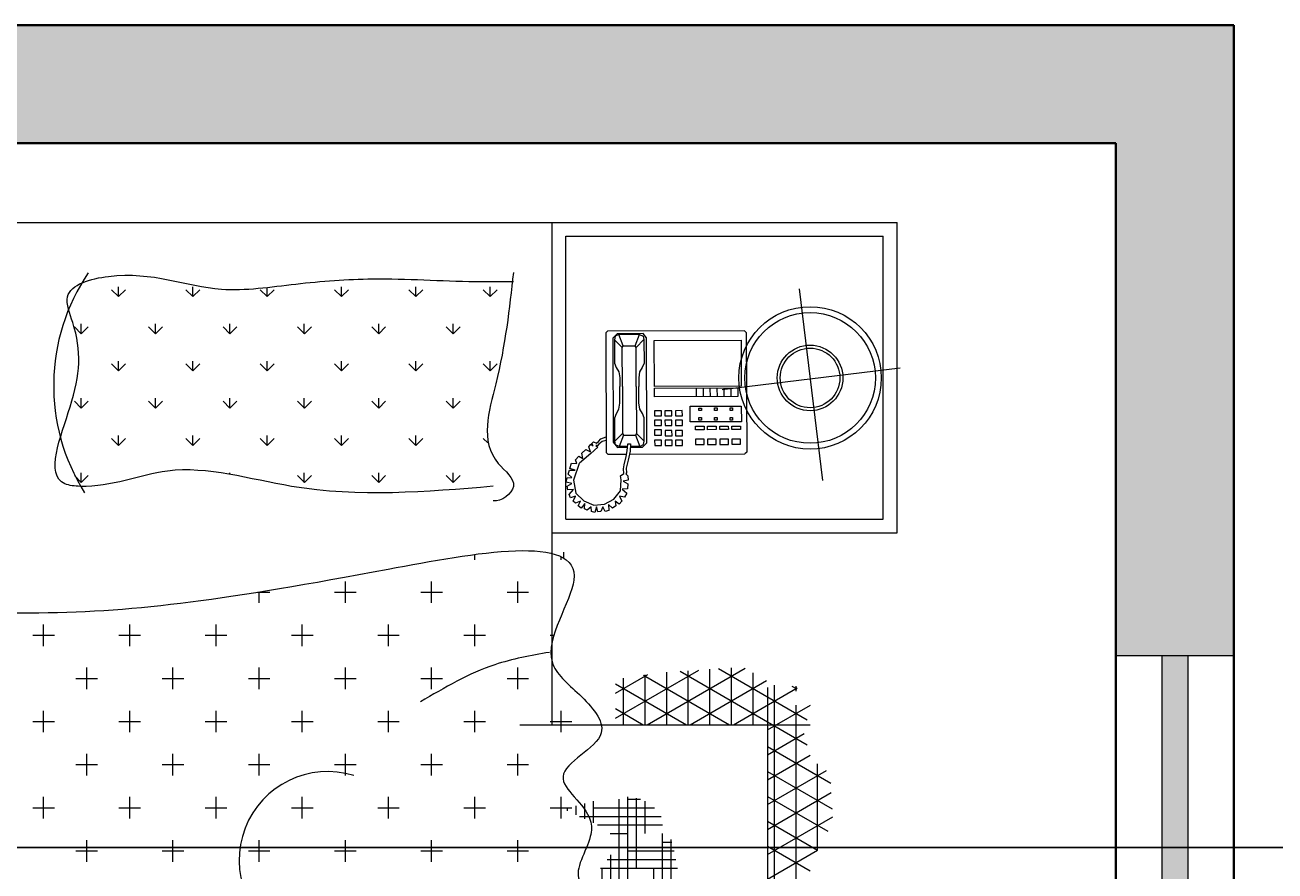
# Model space of a CAD drawing. Units: inches. Extents: x 2330 to 3943, y 1763 to 3461.
# Tile 37 of 40: x 3364 to 3459, y 3098 to 3163. Entities that reach past the tile are written whole.
import ezdxf

# ---------------------------------------------------------------- set-up
doc = ezdxf.new("R2010")
doc.units = ezdxf.units.IN
for name, color, linetype, lineweight in [('A-ANNO-DIMS', 2, 'Continuous', 18), ('A-FURN', 8, 'Continuous', 13), ('A-GLAZ', 4, 'Continuous', 18), ('A-WALL', 7, 'Continuous', 40), ('A-WALL-PATT', 252, 'Continuous', 13)]:
    doc.layers.add(name, color=color, linetype=linetype, lineweight=lineweight)
doc.styles.get("Standard").update_dxf_attribs({"font": 'arial.ttf'})
doc.dimstyles.get("Standard").update_dxf_attribs({"dimtxt": 0.18, "dimasz": 0.18, "dimexe": 0.18, "dimexo": 0.0625, "dimgap": 0.09, "dimtad": 0, "dimtih": 1, "dimtoh": 1, "dimdec": 4, "dimzin": 0, "dimdsep": 46, "dimtxsty": 'Standard', "dimcen": 0.09, "dimadec": 0, "dimazin": 0, "dimtfac": 1, "dimtdec": 4, "dimtofl": 0, "dimtmove": 0, "dimatfit": 3, "dimfxl": 1, "dimtolj": 1, "dimtzin": 0, "dimarcsym": 0})

# ---------------------------------------------------------------- blocks, each defined once
blk = doc.blocks.new('A$C200C7901')
for p, q in [((0.5, 2.3334), (2, 2.3334)), ((2, 2.3334), (2.5, 2.3334)), ((2, 1.6055), (2, 2.3334)), ((2.5, 1.8834), (2.5, 2.3334)), ((1.3176, 2.1721), (1.3075, 2.1822)), ((1.3176, 2.1721), (1.3075, 2.1822)), ((2, 1.8834), (2.5, 1.8834)), ((2.0129, 1.8445), (2.0129, 1.849)), ((2.0129, 1.8445), (2.0129, 1.849)), ((2.0171, 1.8467), (2.0171, 1.8556)), ((2.0171, 1.8467), (2.0171, 1.8556)), ((1.9972, 1.7352), (2.0027, 1.7352)), ((1.9972, 1.7352), (2.0027, 1.7352)), ((2, 1.6963), (2, 1.7248)), ((2, 1.6963), (2, 1.7248)), ((2.3121, 1.6596), (2.3121, 0.0201)), ((1.9533, 1.6055), (2.3741, 1.6055)), ((1.9533, 1.6055), (2.3741, 1.6055))]:
    blk.add_line(p, q)
at = {"linetype": 'ByBlock'}
for p, q in [((2.02, 2.3134), (2.48, 2.3134)), ((2.02, 1.9034), (2.02, 2.3134)), ((2.48, 1.9034), (2.48, 2.3134)), ((1.3714, 2.2259), (1.3613, 2.236)), ((1.3714, 2.2259), (1.3613, 2.236)), ((1.3714, 2.2259), (1.3714, 2.2402)), ((1.3714, 2.2259), (1.3714, 2.2402)), ((1.3714, 2.2259), (1.3815, 2.236)), ((1.3714, 2.2259), (1.3815, 2.236)), ((1.4792, 2.2259), (1.4691, 2.236)), ((1.4792, 2.2259), (1.4691, 2.236)), ((1.4792, 2.2259), (1.4792, 2.2402)), ((1.4792, 2.2259), (1.4792, 2.2402)), ((1.4792, 2.2259), (1.4893, 2.236)), ((1.4792, 2.2259), (1.4893, 2.236)), ((1.587, 2.2259), (1.5769, 2.236)), ((1.587, 2.2259), (1.5769, 2.236)), ((1.587, 2.2259), (1.587, 2.2393)), ((1.587, 2.2259), (1.587, 2.2393)), ((1.587, 2.2259), (1.5971, 2.236)), ((1.587, 2.2259), (1.5971, 2.236)), ((1.6947, 2.2259), (1.6846, 2.236)), ((1.6947, 2.2259), (1.6846, 2.236)), ((1.6947, 2.2259), (1.6947, 2.2402)), ((1.6947, 2.2259), (1.6947, 2.2402)), ((1.6947, 2.2259), (1.7048, 2.236)), ((1.6947, 2.2259), (1.7048, 2.236)), ((1.8025, 2.2259), (1.7924, 2.236)), ((1.8025, 2.2259), (1.7924, 2.236)), ((1.8025, 2.2259), (1.8025, 2.2402)), ((1.8025, 2.2259), (1.8025, 2.2402)), ((1.8025, 2.2259), (1.8126, 2.236)), ((1.8025, 2.2259), (1.8126, 2.236)), ((1.9103, 2.2259), (1.9002, 2.236)), ((1.9103, 2.2259), (1.9002, 2.236)), ((1.9103, 2.2259), (1.9103, 2.2402)), ((1.9103, 2.2259), (1.9103, 2.2402)), ((1.9103, 2.2259), (1.9204, 2.236)), ((1.9103, 2.2259), (1.9204, 2.236)), ((2.3581, 2.2373), (2.3919, 1.9595)), ((1.3176, 2.172), (1.3176, 2.1863)), ((1.3176, 2.172), (1.3176, 2.1863)), ((1.3176, 2.1721), (1.3277, 2.1822)), ((1.3176, 2.1721), (1.3277, 2.1822)), ((1.4253, 2.1721), (1.4152, 2.1822)), ((1.4253, 2.1721), (1.4152, 2.1822)), ((1.4253, 2.172), (1.4253, 2.1863)), ((1.4253, 2.172), (1.4253, 2.1863)), ((1.4253, 2.1721), (1.4354, 2.1822)), ((1.4253, 2.1721), (1.4354, 2.1822)), ((1.5331, 2.1721), (1.523, 2.1822)), ((1.5331, 2.1721), (1.523, 2.1822)), ((1.5331, 2.172), (1.5331, 2.1863)), ((1.5331, 2.172), (1.5331, 2.1863)), ((1.5331, 2.1721), (1.5432, 2.1822)), ((1.5331, 2.1721), (1.5432, 2.1822)), ((1.6409, 2.1721), (1.6308, 2.1822)), ((1.6409, 2.1721), (1.6308, 2.1822)), ((1.6408, 2.172), (1.6408, 2.1863)), ((1.6408, 2.172), (1.6408, 2.1863)), ((1.6409, 2.1721), (1.651, 2.1822)), ((1.6409, 2.1721), (1.651, 2.1822)), ((1.7486, 2.1721), (1.7385, 2.1822)), ((1.7486, 2.1721), (1.7385, 2.1822)), ((1.7486, 2.172), (1.7486, 2.1863)), ((1.7486, 2.172), (1.7486, 2.1863)), ((1.7486, 2.1721), (1.7587, 2.1822)), ((1.7486, 2.1721), (1.7587, 2.1822)), ((1.8564, 2.1721), (1.8463, 2.1822)), ((1.8564, 2.1721), (1.8463, 2.1822)), ((1.8564, 2.172), (1.8564, 2.1863)), ((1.8564, 2.172), (1.8564, 2.1863)), ((1.8564, 2.1721), (1.8665, 2.1822)), ((1.8564, 2.1721), (1.8665, 2.1822)), ((2.0802, 2.176), (2.0777, 2.1734)), ((2.2789, 2.1766), (2.0802, 2.176)), ((2.2789, 2.1766), (2.2814, 2.1741)), ((2.0777, 2.1734), (2.0783, 1.9999)), ((2.0941, 2.1722), (2.0878, 2.1659)), ((2.0878, 2.1659), (2.0883, 2.015)), ((2.0915, 2.1685), (2.0903, 2.1634)), ((2.0903, 2.1634), (2.1017, 2.1521)), ((2.0903, 2.1634), (2.0904, 2.1295)), ((2.0966, 2.171), (2.0915, 2.1685)), ((2.1318, 2.1724), (2.0941, 2.1722)), ((2.1267, 2.1711), (2.0966, 2.171)), ((2.1029, 2.1547), (2.0966, 2.171)), ((2.1205, 2.1547), (2.1267, 2.1711)), ((2.1331, 2.1636), (2.1218, 2.1522)), ((2.1267, 2.1711), (2.1318, 2.1686)), ((2.1368, 2.1661), (2.1318, 2.1724)), ((2.1318, 2.1686), (2.1331, 2.1636)), ((2.1331, 2.1636), (2.1332, 2.1296)), ((2.1373, 2.014), (2.1368, 2.1661)), ((2.1481, 2.1624), (2.2739, 2.1628)), ((2.1484, 2.0957), (2.1481, 2.1624)), ((2.2739, 2.1628), (2.2741, 2.0961)), ((2.2814, 2.1741), (2.282, 2.0006)), ((2.1017, 2.1521), (2.1029, 2.1547)), ((2.1019, 2.0956), (2.1017, 2.1521)), ((2.1029, 2.1547), (2.1205, 2.1547)), ((2.1218, 2.1522), (2.1205, 2.1547)), ((2.122, 2.0956), (2.1218, 2.1522)), ((1.3714, 2.1182), (1.3613, 2.1283)), ((1.3714, 2.1182), (1.3613, 2.1283)), ((1.3714, 2.1182), (1.3714, 2.1325)), ((1.3714, 2.1182), (1.3714, 2.1325)), ((1.3714, 2.1182), (1.3815, 2.1283)), ((1.3714, 2.1182), (1.3815, 2.1283)), ((1.4792, 2.1182), (1.4691, 2.1283)), ((1.4792, 2.1182), (1.4691, 2.1283)), ((1.4792, 2.1182), (1.4792, 2.1325)), ((1.4792, 2.1182), (1.4792, 2.1325)), ((1.4792, 2.1182), (1.4893, 2.1283)), ((1.4792, 2.1182), (1.4893, 2.1283)), ((1.587, 2.1182), (1.5769, 2.1283)), ((1.587, 2.1182), (1.5769, 2.1283)), ((1.587, 2.1182), (1.587, 2.1325)), ((1.587, 2.1182), (1.587, 2.1325)), ((1.587, 2.1182), (1.5971, 2.1283)), ((1.587, 2.1182), (1.5971, 2.1283)), ((1.6947, 2.1182), (1.6846, 2.1283)), ((1.6947, 2.1182), (1.6846, 2.1283)), ((1.6947, 2.1182), (1.6947, 2.1325)), ((1.6947, 2.1182), (1.6947, 2.1325)), ((1.6947, 2.1182), (1.7048, 2.1283)), ((1.6947, 2.1182), (1.7048, 2.1283)), ((1.8025, 2.1182), (1.7924, 2.1283)), ((1.8025, 2.1182), (1.7924, 2.1283)), ((1.8025, 2.1182), (1.8025, 2.1325)), ((1.8025, 2.1182), (1.8025, 2.1325)), ((1.8025, 2.1182), (1.8126, 2.1283)), ((1.8025, 2.1182), (1.8126, 2.1283)), ((1.9103, 2.1182), (1.9002, 2.1283)), ((1.9103, 2.1182), (1.9002, 2.1283)), ((1.9103, 2.1182), (1.9103, 2.1325)), ((1.9103, 2.1182), (1.9103, 2.1325)), ((1.9103, 2.1182), (1.9204, 2.1283)), ((1.9103, 2.1182), (1.9204, 2.1283)), ((2.0904, 2.1295), (2.093, 2.1232)), ((2.093, 2.1232), (2.0968, 2.1169)), ((2.1307, 2.1233), (2.1269, 2.117)), ((2.1332, 2.1296), (2.1307, 2.1233)), ((2.2464, 2.0911), (2.5044, 2.1228)), ((2.0968, 2.1169), (2.098, 2.1081)), ((2.098, 2.1081), (2.0981, 2.0956)), ((2.1269, 2.117), (2.1257, 2.1082)), ((2.1257, 2.1082), (2.1257, 2.0956)), ((2.0982, 2.0717), (2.0981, 2.0956)), ((2.1019, 2.0956), (2.1021, 2.0277)), ((2.122, 2.0956), (2.1222, 2.0277)), ((2.1258, 2.0718), (2.1257, 2.0956)), ((2.2741, 2.0961), (2.1484, 2.0957)), ((2.1484, 2.0932), (2.2691, 2.0936)), ((2.1484, 2.0806), (2.1484, 2.0932)), ((2.2087, 2.0934), (2.2088, 2.0808)), ((2.2188, 2.0934), (2.2188, 2.0809)), ((2.2288, 2.0935), (2.2289, 2.0809)), ((2.2389, 2.0935), (2.239, 2.0809)), ((2.249, 2.0935), (2.249, 2.081)), ((2.259, 2.0936), (2.2591, 2.081)), ((2.2691, 2.0936), (2.2691, 2.081)), ((1.3176, 2.0643), (1.3075, 2.0744)), ((1.3176, 2.0643), (1.3075, 2.0744)), ((1.3176, 2.0643), (1.3176, 2.0786)), ((1.3176, 2.0643), (1.3176, 2.0786)), ((1.3176, 2.0643), (1.3277, 2.0744)), ((1.3176, 2.0643), (1.3277, 2.0744)), ((1.4253, 2.0643), (1.4152, 2.0744)), ((1.4253, 2.0643), (1.4152, 2.0744)), ((1.4253, 2.0643), (1.4253, 2.0786)), ((1.4253, 2.0643), (1.4253, 2.0786)), ((1.4253, 2.0643), (1.4354, 2.0744)), ((1.4253, 2.0643), (1.4354, 2.0744)), ((1.5331, 2.0643), (1.523, 2.0744)), ((1.5331, 2.0643), (1.523, 2.0744)), ((1.5331, 2.0643), (1.5331, 2.0786)), ((1.5331, 2.0643), (1.5331, 2.0786)), ((1.5331, 2.0643), (1.5432, 2.0744)), ((1.5331, 2.0643), (1.5432, 2.0744)), ((1.6409, 2.0643), (1.6308, 2.0744)), ((1.6409, 2.0643), (1.6308, 2.0744)), ((1.6408, 2.0643), (1.6408, 2.0786)), ((1.6408, 2.0643), (1.6408, 2.0786)), ((1.6409, 2.0643), (1.651, 2.0744)), ((1.6409, 2.0643), (1.651, 2.0744)), ((1.7486, 2.0643), (1.7385, 2.0744)), ((1.7486, 2.0643), (1.7385, 2.0744)), ((1.7486, 2.0643), (1.7486, 2.0786)), ((1.7486, 2.0643), (1.7486, 2.0786)), ((1.7486, 2.0643), (1.7587, 2.0744)), ((1.7486, 2.0643), (1.7587, 2.0744)), ((1.8564, 2.0643), (1.8463, 2.0744)), ((1.8564, 2.0643), (1.8463, 2.0744)), ((1.8564, 2.0643), (1.8564, 2.0786)), ((1.8564, 2.0643), (1.8564, 2.0786)), ((1.8564, 2.0643), (1.8665, 2.0744)), ((1.8564, 2.0643), (1.8665, 2.0744)), ((2.0969, 2.0629), (2.0982, 2.0717)), ((2.1271, 2.063), (2.1258, 2.0718)), ((2.2691, 2.081), (2.1484, 2.0806)), ((2.2, 2.067), (2.2742, 2.0672)), ((2.2001, 2.0443), (2.2, 2.067)), ((2.2742, 2.0672), (2.2743, 2.0446)), ((2.0907, 2.0503), (2.0932, 2.0566)), ((2.0908, 2.0163), (2.0907, 2.0503)), ((2.0932, 2.0566), (2.0969, 2.0629)), ((2.1309, 2.0567), (2.1271, 2.063)), ((2.1334, 2.0504), (2.1309, 2.0567)), ((2.1336, 2.0165), (2.1334, 2.0504)), ((2.1586, 2.0606), (2.1485, 2.0605)), ((2.1485, 2.0605), (2.1485, 2.053)), ((2.1485, 2.053), (2.1586, 2.053)), ((2.1586, 2.053), (2.1586, 2.0606)), ((2.1636, 2.0606), (2.1636, 2.053)), ((2.1736, 2.0606), (2.1636, 2.0606)), ((2.1636, 2.053), (2.1737, 2.0531)), ((2.1737, 2.0531), (2.1736, 2.0606)), ((2.1887, 2.0607), (2.1787, 2.0606)), ((2.1787, 2.0606), (2.1787, 2.0531)), ((2.1787, 2.0531), (2.1888, 2.0531)), ((2.1888, 2.0531), (2.1887, 2.0607)), ((2.2126, 2.0645), (2.2164, 2.0645)), ((2.2126, 2.0607), (2.2126, 2.0645)), ((2.2164, 2.0607), (2.2126, 2.0607)), ((2.2126, 2.0507), (2.2164, 2.0507)), ((2.2127, 2.0469), (2.2126, 2.0507)), ((2.2164, 2.0645), (2.2164, 2.0607)), ((2.2164, 2.0507), (2.2164, 2.0469)), ((2.2352, 2.0646), (2.239, 2.0646)), ((2.2352, 2.0608), (2.2352, 2.0646)), ((2.239, 2.0608), (2.2352, 2.0608)), ((2.2353, 2.0508), (2.2391, 2.0508)), ((2.2353, 2.047), (2.2353, 2.0508)), ((2.239, 2.0646), (2.239, 2.0608)), ((2.2391, 2.0508), (2.2391, 2.047)), ((2.2579, 2.0609), (2.2579, 2.0647)), ((2.2579, 2.0647), (2.2616, 2.0647)), ((2.2616, 2.0609), (2.2579, 2.0609)), ((2.2579, 2.0508), (2.2617, 2.0508)), ((2.2579, 2.0471), (2.2579, 2.0508)), ((2.2616, 2.0647), (2.2616, 2.0609)), ((2.2617, 2.0508), (2.2617, 2.0471)), ((2.1485, 2.0467), (2.1486, 2.0391)), ((2.1586, 2.0467), (2.1485, 2.0467)), ((2.1486, 2.0391), (2.1586, 2.0392)), ((2.1586, 2.0329), (2.1486, 2.0329)), ((2.1486, 2.0329), (2.1486, 2.0253)), ((2.1586, 2.0392), (2.1586, 2.0467)), ((2.1587, 2.0253), (2.1586, 2.0329)), ((2.1737, 2.0468), (2.1636, 2.0467)), ((2.1636, 2.0467), (2.1637, 2.0392)), ((2.1637, 2.0392), (2.1737, 2.0392)), ((2.1637, 2.0317), (2.1637, 2.0241)), ((2.1737, 2.0317), (2.1637, 2.0317)), ((2.1737, 2.0392), (2.1737, 2.0468)), ((2.1738, 2.0241), (2.1737, 2.0317)), ((2.1787, 2.0468), (2.1787, 2.0392)), ((2.1888, 2.0468), (2.1787, 2.0468)), ((2.1787, 2.0392), (2.1888, 2.0393)), ((2.1788, 2.0317), (2.1788, 2.0242)), ((2.1888, 2.0317), (2.1788, 2.0317)), ((2.1888, 2.0393), (2.1888, 2.0468)), ((2.1889, 2.0242), (2.1888, 2.0317)), ((2.2743, 2.0446), (2.2001, 2.0443)), ((2.2077, 2.0331), (2.2077, 2.0381)), ((2.2077, 2.0381), (2.2202, 2.0381)), ((2.2203, 2.0331), (2.2077, 2.0331)), ((2.2164, 2.0469), (2.2127, 2.0469)), ((2.2202, 2.0381), (2.2203, 2.0331)), ((2.2253, 2.0381), (2.2378, 2.0382)), ((2.2253, 2.0331), (2.2253, 2.0381)), ((2.2379, 2.0332), (2.2253, 2.0331)), ((2.2391, 2.047), (2.2353, 2.047)), ((2.2378, 2.0382), (2.2379, 2.0332)), ((2.2429, 2.0332), (2.2429, 2.0382)), ((2.2429, 2.0382), (2.2554, 2.0382)), ((2.2555, 2.0332), (2.2429, 2.0332)), ((2.2554, 2.0382), (2.2555, 2.0332)), ((2.2617, 2.0471), (2.2579, 2.0471)), ((2.2605, 2.0332), (2.2605, 2.0383)), ((2.2605, 2.0383), (2.273, 2.0383)), ((2.2731, 2.0333), (2.2605, 2.0332)), ((2.273, 2.0383), (2.2731, 2.0333)), ((1.3714, 2.0104), (1.3613, 2.0205)), ((1.3714, 2.0104), (1.3613, 2.0205)), ((1.3714, 2.0104), (1.3714, 2.0247)), ((1.3714, 2.0104), (1.3714, 2.0247)), ((1.3714, 2.0104), (1.3815, 2.0205)), ((1.3714, 2.0104), (1.3815, 2.0205)), ((1.4792, 2.0104), (1.4691, 2.0205)), ((1.4792, 2.0104), (1.4691, 2.0205)), ((1.4792, 2.0104), (1.4792, 2.0247)), ((1.4792, 2.0104), (1.4792, 2.0247)), ((1.4792, 2.0104), (1.4893, 2.0205)), ((1.4792, 2.0104), (1.4893, 2.0205)), ((1.587, 2.0104), (1.5769, 2.0205)), ((1.587, 2.0104), (1.5769, 2.0205)), ((1.587, 2.0104), (1.587, 2.0247)), ((1.587, 2.0104), (1.587, 2.0247)), ((1.587, 2.0104), (1.5971, 2.0205)), ((1.587, 2.0104), (1.5971, 2.0205)), ((1.6947, 2.0104), (1.6846, 2.0205)), ((1.6947, 2.0104), (1.6846, 2.0205)), ((1.6947, 2.0104), (1.6947, 2.0247)), ((1.6947, 2.0104), (1.6947, 2.0247)), ((1.6947, 2.0104), (1.7048, 2.0205)), ((1.6947, 2.0104), (1.7048, 2.0205)), ((1.8025, 2.0104), (1.7924, 2.0205)), ((1.8025, 2.0104), (1.7924, 2.0205)), ((1.8025, 2.0104), (1.8025, 2.0247)), ((1.8025, 2.0104), (1.8025, 2.0247)), ((1.8025, 2.0104), (1.8126, 2.0205)), ((1.8025, 2.0104), (1.8126, 2.0205)), ((1.9068, 2.0139), (1.9002, 2.0205)), ((1.9068, 2.0139), (1.9002, 2.0205)), ((2.053, 2.0084), (2.0563, 2.0119)), ((2.0563, 2.0119), (2.0594, 2.0095)), ((2.0576, 2.0133), (2.0598, 2.0155)), ((2.0594, 2.0095), (2.0576, 2.0133)), ((2.0598, 2.0155), (2.0645, 2.0137)), ((2.0645, 2.0137), (2.0671, 2.0162)), ((2.0676, 2.012), (2.0663, 2.0102)), ((2.0671, 2.0162), (2.0707, 2.0197)), ((2.0727, 2.016), (2.0676, 2.012)), ((2.0707, 2.0197), (2.0782, 2.0226)), ((2.0782, 2.0175), (2.0727, 2.016)), ((2.0883, 2.015), (2.0946, 2.0075)), ((2.0908, 2.0163), (2.1021, 2.0277)), ((2.0921, 2.0113), (2.0908, 2.0163)), ((2.0971, 2.0088), (2.0921, 2.0113)), ((2.1034, 2.0252), (2.0971, 2.0088)), ((2.1021, 2.0277), (2.1034, 2.0252)), ((2.1034, 2.0252), (2.121, 2.0252)), ((2.109, 2.0025), (2.1097, 2.0126)), ((2.1097, 2.0126), (2.1135, 2.0126)), ((2.1135, 2.0126), (2.1133, 2.0018)), ((2.1222, 2.0277), (2.121, 2.0252)), ((2.121, 2.0252), (2.1273, 2.0089)), ((2.1336, 2.0165), (2.1222, 2.0277)), ((2.1273, 2.0089), (2.1323, 2.0114)), ((2.1311, 2.0077), (2.1373, 2.014)), ((2.1323, 2.0114), (2.1336, 2.0165)), ((2.1486, 2.0253), (2.1587, 2.0253)), ((2.1587, 2.0178), (2.1486, 2.0178)), ((2.1486, 2.0178), (2.1487, 2.0102)), ((2.1587, 2.0103), (2.1587, 2.0178)), ((2.1637, 2.0241), (2.1738, 2.0241)), ((2.1738, 2.0179), (2.1637, 2.0178)), ((2.1637, 2.0178), (2.1638, 2.0103)), ((2.1738, 2.0103), (2.1738, 2.0179)), ((2.1788, 2.0242), (2.1889, 2.0242)), ((2.1788, 2.0179), (2.1788, 2.0103)), ((2.1889, 2.0179), (2.1788, 2.0179)), ((2.1889, 2.0104), (2.1889, 2.0179)), ((2.2203, 2.0193), (2.2077, 2.0192)), ((2.2077, 2.0192), (2.2078, 2.0117)), ((2.2078, 2.0117), (2.2203, 2.0117)), ((2.2203, 2.0117), (2.2203, 2.0193)), ((2.2379, 2.0193), (2.2253, 2.0193)), ((2.2253, 2.0193), (2.2254, 2.0117)), ((2.2254, 2.0117), (2.2379, 2.0118)), ((2.2379, 2.0118), (2.2379, 2.0193)), ((2.2555, 2.0194), (2.2429, 2.0193)), ((2.2429, 2.0193), (2.243, 2.0118)), ((2.243, 2.0118), (2.2555, 2.0118)), ((2.2555, 2.0118), (2.2555, 2.0194)), ((2.2605, 2.0194), (2.2606, 2.0119)), ((2.2731, 2.0194), (2.2605, 2.0194)), ((2.2606, 2.0119), (2.2731, 2.0119)), ((2.2731, 2.0119), (2.2731, 2.0194)), ((2.0338, 1.9895), (2.0386, 1.9946)), ((2.0386, 1.9946), (2.0444, 1.9911)), ((2.0561, 1.9986), (2.0396, 1.9844)), ((2.0431, 1.999), (2.0488, 2.0046)), ((2.0444, 1.9911), (2.0431, 1.999)), ((2.0488, 2.0046), (2.0557, 2.0011)), ((2.0557, 2.0011), (2.053, 2.0084)), ((2.0663, 2.0077), (2.0561, 1.9986)), ((2.0663, 2.0102), (2.0636, 2.0104)), ((2.0636, 2.0104), (2.0663, 2.0077)), ((2.0783, 1.9999), (2.0808, 1.9974)), ((2.0808, 1.9974), (2.1079, 1.9975)), ((2.0946, 2.0075), (2.1093, 2.0076)), ((2.1094, 2.0088), (2.0971, 2.0088)), ((2.1042, 1.9824), (2.1072, 1.9944)), ((2.1072, 1.9944), (2.109, 2.0025)), ((2.1133, 2.0018), (2.1103, 1.989)), ((2.1123, 1.9975), (2.2795, 1.9981)), ((2.1273, 2.0089), (2.1134, 2.0088)), ((2.1134, 2.0076), (2.1311, 2.0077)), ((2.1487, 2.0102), (2.1587, 2.0103)), ((2.1638, 2.0103), (2.1738, 2.0103)), ((2.1788, 2.0103), (2.1889, 2.0104)), ((2.282, 2.0006), (2.2795, 1.9981)), ((2.0259, 1.977), (2.0281, 1.9847)), ((2.0333, 1.9743), (2.0259, 1.977)), ((2.0281, 1.9847), (2.0358, 1.9839)), ((2.0393, 1.984), (2.031, 1.96)), ((2.0358, 1.9839), (2.0338, 1.9895)), ((2.1035, 1.9763), (2.1042, 1.9824)), ((2.1038, 1.9697), (2.1035, 1.9763)), ((2.1103, 1.989), (2.1073, 1.9771)), ((2.1073, 1.9771), (2.1076, 1.9704)), ((1.3176, 1.9565), (1.3075, 1.9666)), ((1.3176, 1.9565), (1.3075, 1.9666)), ((1.3176, 1.9565), (1.3176, 1.9708)), ((1.3176, 1.9565), (1.3176, 1.9708)), ((1.3176, 1.9565), (1.3277, 1.9666)), ((1.3176, 1.9565), (1.3277, 1.9666)), ((1.4253, 1.9703), (1.4253, 1.9708)), ((1.4253, 1.9703), (1.4253, 1.9708)), ((1.5331, 1.9683), (1.5331, 1.9708)), ((1.5331, 1.9683), (1.5331, 1.9708)), ((1.543, 1.9665), (1.5432, 1.9666)), ((1.543, 1.9665), (1.5432, 1.9666)), ((1.6409, 1.9565), (1.6308, 1.9666)), ((1.6409, 1.9565), (1.6308, 1.9666)), ((1.6408, 1.9565), (1.6408, 1.9708)), ((1.6408, 1.9565), (1.6408, 1.9708)), ((1.6409, 1.9565), (1.651, 1.9666)), ((1.6409, 1.9565), (1.651, 1.9666)), ((1.7486, 1.9565), (1.7385, 1.9666)), ((1.7486, 1.9565), (1.7385, 1.9666)), ((1.7486, 1.9565), (1.7486, 1.9708)), ((1.7486, 1.9565), (1.7486, 1.9708)), ((1.7486, 1.9565), (1.7587, 1.9666)), ((1.7486, 1.9565), (1.7587, 1.9666)), ((1.8564, 1.9565), (1.8463, 1.9666)), ((1.8564, 1.9565), (1.8463, 1.9666)), ((1.8564, 1.9565), (1.8564, 1.9708)), ((1.8564, 1.9565), (1.8564, 1.9708)), ((1.8564, 1.9565), (1.8665, 1.9666)), ((1.8564, 1.9565), (1.8665, 1.9666)), ((2.0206, 1.9572), (2.0218, 1.9635)), ((2.0285, 1.9549), (2.0206, 1.9572)), ((2.0218, 1.9635), (2.0287, 1.9636)), ((2.0234, 1.9686), (2.0251, 1.9745)), ((2.0287, 1.9636), (2.0234, 1.9686)), ((2.0251, 1.9745), (2.0333, 1.9743)), ((2.031, 1.96), (2.0346, 1.9409)), ((2.099, 1.9444), (2.1002, 1.9605)), ((2.0992, 1.9663), (2.1038, 1.9697)), ((2.1002, 1.9605), (2.0992, 1.9663)), ((2.1101, 1.96), (2.1028, 1.9587)), ((2.1028, 1.9587), (2.1099, 1.9544)), ((2.1076, 1.9704), (2.1068, 1.9689)), ((2.1068, 1.9689), (2.1096, 1.9661)), ((2.1096, 1.9661), (2.1101, 1.96)), ((2.0219, 1.9511), (2.0285, 1.9549)), ((2.0229, 1.946), (2.0219, 1.9511)), ((2.0308, 1.9462), (2.0229, 1.946)), ((2.0247, 1.9394), (2.0308, 1.9462)), ((2.0268, 1.9343), (2.0247, 1.9394)), ((2.0346, 1.9409), (2.0459, 1.93)), ((2.0894, 1.9322), (2.099, 1.9444)), ((2.1094, 1.9475), (2.1013, 1.9467)), ((2.1013, 1.9467), (2.1084, 1.9412)), ((2.1084, 1.9412), (2.1051, 1.9353)), ((2.1099, 1.9544), (2.1094, 1.9475)), ((2.0341, 1.9366), (2.0268, 1.9343)), ((2.0306, 1.9297), (2.0341, 1.9366)), ((2.0339, 1.9267), (2.0306, 1.9297)), ((2.041, 1.9297), (2.0339, 1.9267)), ((2.038, 1.9228), (2.041, 1.9297)), ((2.0421, 1.9193), (2.038, 1.9228)), ((2.0474, 1.9259), (2.0421, 1.9193)), ((2.0459, 1.93), (2.0607, 1.9237)), ((2.0467, 1.9183), (2.0474, 1.9259)), ((2.0566, 1.9214), (2.0508, 1.9163)), ((2.0569, 1.9145), (2.0566, 1.9214)), ((2.0607, 1.9237), (2.0759, 1.925)), ((2.0645, 1.9214), (2.0617, 1.9133)), ((2.0663, 1.914), (2.0645, 1.9214)), ((2.0736, 1.9214), (2.0706, 1.9146)), ((2.077, 1.9146), (2.0736, 1.9214)), ((2.0759, 1.925), (2.0894, 1.9322)), ((2.0876, 1.9195), (2.0815, 1.9245)), ((2.0815, 1.9245), (2.0823, 1.9161)), ((2.0925, 1.9225), (2.0876, 1.9195)), ((2.0973, 1.9251), (2.0914, 1.9294)), ((2.0914, 1.9294), (2.0925, 1.9225)), ((2.1011, 1.9297), (2.0973, 1.9251)), ((2.1051, 1.9353), (2.0975, 1.9368)), ((2.0975, 1.9368), (2.1011, 1.9297)), ((2.02, 1.9034), (2.48, 1.9034)), ((2.0508, 1.9163), (2.0467, 1.9183)), ((2.0617, 1.9133), (2.0569, 1.9145)), ((2.0706, 1.9146), (2.0663, 1.914)), ((2.0823, 1.9161), (2.077, 1.9146)), ((1.8879, 1.8445), (1.8879, 1.8523)), ((1.8879, 1.8445), (1.8879, 1.8523)), ((1.7004, 1.782), (1.7004, 1.8133)), ((1.7004, 1.782), (1.7004, 1.8133)), ((1.8254, 1.782), (1.8254, 1.8133)), ((1.8254, 1.782), (1.8254, 1.8133)), ((1.9504, 1.782), (1.9504, 1.8133)), ((1.9504, 1.782), (1.9504, 1.8133)), ((1.573, 1.7977), (1.591, 1.7977)), ((1.573, 1.7977), (1.591, 1.7977)), ((1.5754, 1.782), (1.5754, 1.7981)), ((1.5754, 1.782), (1.5754, 1.7981)), ((1.6847, 1.7977), (1.716, 1.7977)), ((1.6847, 1.7977), (1.716, 1.7977)), ((1.8097, 1.7977), (1.841, 1.7977)), ((1.8097, 1.7977), (1.841, 1.7977)), ((1.9347, 1.7977), (1.966, 1.7977)), ((1.9347, 1.7977), (1.966, 1.7977)), ((1.2629, 1.7195), (1.2629, 1.7508)), ((1.2629, 1.7195), (1.2629, 1.7508)), ((1.3879, 1.7195), (1.3879, 1.7508)), ((1.3879, 1.7195), (1.3879, 1.7508)), ((1.5129, 1.7195), (1.5129, 1.7508)), ((1.5129, 1.7195), (1.5129, 1.7508)), ((1.6379, 1.7195), (1.6379, 1.7508)), ((1.6379, 1.7195), (1.6379, 1.7508)), ((1.7629, 1.7195), (1.7629, 1.7508)), ((1.7629, 1.7195), (1.7629, 1.7508)), ((1.8879, 1.7195), (1.8879, 1.7508)), ((1.8879, 1.7195), (1.8879, 1.7508)), ((1.2472, 1.7352), (1.2785, 1.7352)), ((1.2472, 1.7352), (1.2785, 1.7352)), ((1.3722, 1.7352), (1.4035, 1.7352)), ((1.3722, 1.7352), (1.4035, 1.7352)), ((1.4972, 1.7352), (1.5285, 1.7352)), ((1.4972, 1.7352), (1.5285, 1.7352)), ((1.6222, 1.7352), (1.6535, 1.7352)), ((1.6222, 1.7352), (1.6535, 1.7352)), ((1.7472, 1.7352), (1.7785, 1.7352)), ((1.7472, 1.7352), (1.7785, 1.7352)), ((1.8722, 1.7352), (1.9035, 1.7352)), ((1.8722, 1.7352), (1.9035, 1.7352)), ((1.3254, 1.657), (1.3254, 1.6883)), ((1.3254, 1.657), (1.3254, 1.6883)), ((1.4504, 1.657), (1.4504, 1.6883)), ((1.4504, 1.657), (1.4504, 1.6883)), ((1.5754, 1.657), (1.5754, 1.6883)), ((1.5754, 1.657), (1.5754, 1.6883)), ((1.7004, 1.657), (1.7004, 1.6883)), ((1.7004, 1.657), (1.7004, 1.6883)), ((1.8254, 1.657), (1.8254, 1.6883)), ((1.8254, 1.657), (1.8254, 1.6883)), ((1.9504, 1.657), (1.9504, 1.6883)), ((1.9504, 1.657), (1.9504, 1.6883)), ((2.1377, 1.6055), (2.2798, 1.6876)), ((2.1377, 1.6055), (2.2798, 1.6876)), ((2.2287, 1.6055), (2.2287, 1.6859)), ((2.2287, 1.6055), (2.2287, 1.6859)), ((2.2414, 1.6868), (2.3699, 1.6126)), ((2.2414, 1.6868), (2.3699, 1.6126)), ((2.2599, 1.6055), (2.2599, 1.688)), ((2.2599, 1.6055), (2.2599, 1.688)), ((1.3097, 1.6727), (1.341, 1.6727)), ((1.3097, 1.6727), (1.341, 1.6727)), ((1.4347, 1.6727), (1.466, 1.6727)), ((1.4347, 1.6727), (1.466, 1.6727)), ((1.5597, 1.6727), (1.591, 1.6727)), ((1.5597, 1.6727), (1.591, 1.6727)), ((1.6847, 1.6727), (1.716, 1.6727)), ((1.6847, 1.6727), (1.716, 1.6727)), ((1.8097, 1.6727), (1.841, 1.6727)), ((1.8097, 1.6727), (1.841, 1.6727)), ((1.9347, 1.6727), (1.966, 1.6727)), ((1.9347, 1.6727), (1.966, 1.6727)), ((2.0919, 1.6152), (2.2125, 1.6848)), ((2.0919, 1.6152), (2.2125, 1.6848)), ((2.0919, 1.6513), (2.1386, 1.6782)), ((2.0919, 1.6513), (2.1386, 1.6782)), ((2.1037, 1.6055), (2.1037, 1.673)), ((2.1037, 1.6055), (2.1037, 1.673)), ((2.1327, 1.6773), (2.2571, 1.6055)), ((2.1327, 1.6773), (2.2571, 1.6055)), ((2.1349, 1.6055), (2.1349, 1.6777)), ((2.1349, 1.6055), (2.1349, 1.6777)), ((2.1662, 1.6055), (2.1662, 1.6817)), ((2.1662, 1.6055), (2.1662, 1.6817)), ((2.1854, 1.683), (2.3697, 1.5766)), ((2.1854, 1.683), (2.3697, 1.5766)), ((2.1974, 1.6055), (2.1974, 1.6838)), ((2.1974, 1.6055), (2.1974, 1.6838)), ((2.2002, 1.6055), (2.3109, 1.6694)), ((2.2002, 1.6055), (2.3109, 1.6694)), ((2.2912, 1.6055), (2.2912, 1.6809)), ((2.2912, 1.6055), (2.2912, 1.6809)), ((2.0919, 1.6649), (2.1946, 1.6055)), ((2.0919, 1.6649), (2.1946, 1.6055)), ((2.2627, 1.6055), (2.3551, 1.6589)), ((2.2627, 1.6055), (2.3551, 1.6589)), ((2.3224, 0.0468), (2.3224, 1.6627)), ((2.3224, 0.0468), (2.3224, 1.6627)), ((2.3476, 1.6616), (2.3547, 1.6575)), ((2.3476, 1.6616), (2.3547, 1.6575)), ((2.3537, 1.6539), (2.3537, 1.6616)), ((2.3537, 1.6539), (2.3537, 1.6616)), ((2.3121, 1.598), (2.3745, 1.634)), ((2.3121, 1.598), (2.3745, 1.634)), ((2.3537, 0.0056), (2.3537, 1.634)), ((2.3537, 0.0056), (2.3537, 1.634)), ((1.2629, 1.5945), (1.2629, 1.6258)), ((1.2629, 1.5945), (1.2629, 1.6258)), ((1.3879, 1.5945), (1.3879, 1.6258)), ((1.3879, 1.5945), (1.3879, 1.6258)), ((1.5129, 1.5945), (1.5129, 1.6258)), ((1.5129, 1.5945), (1.5129, 1.6258)), ((1.6379, 1.5945), (1.6379, 1.6258)), ((1.6379, 1.5945), (1.6379, 1.6258)), ((1.7629, 1.5945), (1.7629, 1.6258)), ((1.7629, 1.5945), (1.7629, 1.6258)), ((1.8879, 1.5945), (1.8879, 1.6258)), ((1.8879, 1.5945), (1.8879, 1.6258)), ((2.0129, 1.5945), (2.0129, 1.6258)), ((2.0129, 1.5945), (2.0129, 1.6258)), ((2.0919, 1.6288), (2.1321, 1.6055)), ((2.0919, 1.6288), (2.1321, 1.6055)), ((1.2472, 1.6102), (1.2785, 1.6102)), ((1.2472, 1.6102), (1.2785, 1.6102)), ((1.3722, 1.6102), (1.4035, 1.6102)), ((1.3722, 1.6102), (1.4035, 1.6102)), ((1.4972, 1.6102), (1.5285, 1.6102)), ((1.4972, 1.6102), (1.5285, 1.6102)), ((1.6222, 1.6102), (1.6535, 1.6102)), ((1.6222, 1.6102), (1.6535, 1.6102)), ((1.7472, 1.6102), (1.7785, 1.6102)), ((1.7472, 1.6102), (1.7785, 1.6102)), ((1.8722, 1.6102), (1.9035, 1.6102)), ((1.8722, 1.6102), (1.9035, 1.6102)), ((1.9972, 1.6102), (2.0285, 1.6102)), ((1.9972, 1.6102), (2.0285, 1.6102)), ((2.3121, 1.5619), (2.3654, 1.5926)), ((2.3121, 1.5619), (2.3654, 1.5926)), ((1.3254, 1.532), (1.3254, 1.5633)), ((1.3254, 1.532), (1.3254, 1.5633)), ((1.4504, 1.532), (1.4504, 1.5633)), ((1.4504, 1.532), (1.4504, 1.5633)), ((1.5754, 1.532), (1.5754, 1.5633)), ((1.5754, 1.532), (1.5754, 1.5633)), ((1.7004, 1.532), (1.7004, 1.5633)), ((1.7004, 1.532), (1.7004, 1.5633)), ((1.8254, 1.532), (1.8254, 1.5633)), ((1.8254, 1.532), (1.8254, 1.5633)), ((1.9504, 1.532), (1.9504, 1.5633)), ((1.9504, 1.532), (1.9504, 1.5633)), ((2.3121, 1.5738), (2.404, 1.5208)), ((2.3121, 1.5738), (2.404, 1.5208)), ((2.3121, 1.5258), (2.3739, 1.5615)), ((2.3121, 1.5258), (2.3739, 1.5615)), ((1.3097, 1.5477), (1.341, 1.5477)), ((1.3097, 1.5477), (1.341, 1.5477)), ((1.4347, 1.5477), (1.466, 1.5477)), ((1.4347, 1.5477), (1.466, 1.5477)), ((1.5597, 1.5477), (1.591, 1.5477)), ((1.5597, 1.5477), (1.591, 1.5477)), ((1.6847, 1.5477), (1.716, 1.5477)), ((1.6847, 1.5477), (1.716, 1.5477)), ((1.8097, 1.5477), (1.841, 1.5477)), ((1.8097, 1.5477), (1.841, 1.5477)), ((1.9347, 1.5477), (1.966, 1.5477)), ((1.9347, 1.5477), (1.966, 1.5477)), ((2.3849, 1.4236), (2.3849, 1.5486)), ((2.3849, 1.4236), (2.3849, 1.5486)), ((2.3121, 1.4897), (2.3979, 1.5393)), ((2.3121, 1.4897), (2.3979, 1.5393)), ((2.3121, 1.5377), (2.406, 1.4835)), ((2.3121, 1.5377), (2.406, 1.4835)), ((2.3121, 1.4537), (2.4047, 1.5071)), ((2.3121, 1.4537), (2.4047, 1.5071)), ((1.2629, 1.4695), (1.2629, 1.5008)), ((1.2629, 1.4695), (1.2629, 1.5008)), ((1.3879, 1.4695), (1.3879, 1.5008)), ((1.3879, 1.4695), (1.3879, 1.5008)), ((1.5129, 1.4695), (1.5129, 1.5008)), ((1.5129, 1.4695), (1.5129, 1.5008)), ((1.6379, 1.4695), (1.6379, 1.5008)), ((1.6379, 1.4695), (1.6379, 1.5008)), ((1.7629, 1.4695), (1.7629, 1.5008)), ((1.7629, 1.4695), (1.7629, 1.5008)), ((1.8879, 1.4695), (1.8879, 1.5008)), ((1.8879, 1.4695), (1.8879, 1.5008)), ((2.0129, 1.4695), (2.0129, 1.5008)), ((2.0129, 1.4695), (2.0129, 1.5008)), ((2.0349, 1.4748), (2.0349, 1.4879)), ((2.0349, 1.4748), (2.0349, 1.4879)), ((2.0474, 1.4691), (2.0474, 1.4915)), ((2.0474, 1.4691), (2.0474, 1.4915)), ((2.0599, 1.4631), (2.0599, 1.4948)), ((2.0599, 1.4631), (2.0599, 1.4948)), ((2.0974, 1.2977), (2.0974, 1.4977)), ((2.0974, 1.2977), (2.0974, 1.4977)), ((2.1099, 1.3477), (2.1099, 1.5009)), ((2.1099, 1.3477), (2.1099, 1.5009)), ((2.1099, 1.4977), (2.1279, 1.4977)), ((2.1099, 1.4977), (2.1279, 1.4977)), ((2.1224, 1.3977), (2.1224, 1.4992)), ((2.1224, 1.3977), (2.1224, 1.4992)), ((2.1349, 1.4477), (2.1349, 1.4949)), ((2.1349, 1.4477), (2.1349, 1.4949)), ((2.3121, 1.5016), (2.3997, 1.4511)), ((2.3121, 1.5016), (2.3997, 1.4511)), ((1.2472, 1.4852), (1.2785, 1.4852)), ((1.2472, 1.4852), (1.2785, 1.4852)), ((1.3722, 1.4852), (1.4035, 1.4852)), ((1.3722, 1.4852), (1.4035, 1.4852)), ((1.4972, 1.4852), (1.5285, 1.4852)), ((1.4972, 1.4852), (1.5285, 1.4852)), ((1.6222, 1.4852), (1.6535, 1.4852)), ((1.6222, 1.4852), (1.6535, 1.4852)), ((1.7472, 1.4852), (1.7785, 1.4852)), ((1.7472, 1.4852), (1.7785, 1.4852)), ((1.8722, 1.4852), (1.9035, 1.4852)), ((1.8722, 1.4852), (1.9035, 1.4852)), ((1.9972, 1.4852), (2.0285, 1.4852)), ((1.9972, 1.4852), (2.0285, 1.4852)), ((2.0224, 1.4805), (2.0224, 1.4839)), ((2.0224, 1.4805), (2.0224, 1.4839)), ((2.0397, 1.4727), (2.1581, 1.4727)), ((2.0397, 1.4727), (2.1581, 1.4727)), ((2.0599, 1.4852), (2.1484, 1.4852)), ((2.0599, 1.4852), (2.1484, 1.4852)), ((2.3121, 1.4176), (2.4067, 1.4721)), ((2.3121, 1.4176), (2.4067, 1.4721)), ((2.0656, 1.4602), (2.1599, 1.4602)), ((2.0656, 1.4602), (2.1599, 1.4602)), ((2.3121, 1.4655), (2.3849, 1.4235)), ((2.3121, 1.4655), (2.3849, 1.4235)), ((1.3254, 1.407), (1.3254, 1.4383)), ((1.3254, 1.407), (1.3254, 1.4383)), ((1.4504, 1.407), (1.4504, 1.4383)), ((1.4504, 1.407), (1.4504, 1.4383)), ((1.5754, 1.407), (1.5754, 1.4383)), ((1.5754, 1.407), (1.5754, 1.4383)), ((1.7004, 1.407), (1.7004, 1.4383)), ((1.7004, 1.407), (1.7004, 1.4383)), ((1.8254, 1.407), (1.8254, 1.4383)), ((1.8254, 1.407), (1.8254, 1.4383)), ((1.9504, 1.407), (1.9504, 1.4383)), ((1.9504, 1.407), (1.9504, 1.4383)), ((2.084, 1.4477), (2.1099, 1.4477)), ((2.084, 1.4477), (2.1099, 1.4477)), ((2.0849, 1.4468), (2.0849, 1.4477)), ((2.0849, 1.4468), (2.0849, 1.4477)), ((2.1599, 1.2477), (2.1599, 1.4477)), ((2.1599, 1.2477), (2.1599, 1.4477)), ((2.1599, 1.4352), (2.1735, 1.4352)), ((2.1599, 1.4352), (2.1735, 1.4352)), ((2.1724, 1.2977), (2.1724, 1.439)), ((2.1724, 1.2977), (2.1724, 1.439)), ((1.3097, 1.4227), (1.341, 1.4227)), ((1.3097, 1.4227), (1.341, 1.4227)), ((1.4347, 1.4227), (1.466, 1.4227)), ((1.4347, 1.4227), (1.466, 1.4227)), ((1.5597, 1.4227), (1.591, 1.4227)), ((1.5597, 1.4227), (1.591, 1.4227)), ((1.6847, 1.4227), (1.716, 1.4227)), ((1.6847, 1.4227), (1.716, 1.4227)), ((1.8097, 1.4227), (1.841, 1.4227)), ((1.8097, 1.4227), (1.841, 1.4227)), ((1.9347, 1.4227), (1.966, 1.4227)), ((1.9347, 1.4227), (1.966, 1.4227)), ((2.0849, 1.2477), (2.0849, 1.4171)), ((2.0849, 1.2477), (2.0849, 1.4171)), ((2.1099, 1.4227), (2.1767, 1.4227)), ((2.1099, 1.4227), (2.1767, 1.4227)), ((2.3121, 1.4294), (2.3741, 1.3937)), ((2.3121, 1.4294), (2.3741, 1.3937)), ((2.3121, 1.3815), (2.3848, 1.4235)), ((2.3121, 1.3815), (2.3848, 1.4235)), ((2.0703, 1.3977), (2.1819, 1.3977)), ((2.0703, 1.3977), (2.1819, 1.3977)), ((2.0724, 1.1977), (2.0724, 1.3977)), ((2.0724, 1.1977), (2.0724, 1.3977)), ((2.08, 1.4102), (2.1795, 1.4102)), ((2.08, 1.4102), (2.1795, 1.4102)), ((2.1474, 1.1977), (2.1474, 1.3977)), ((2.1474, 1.1977), (2.1474, 1.3977))]:
    blk.add_line(p, q, dxfattribs=at)
for radius in [0.1032, 0.0947, 0.0475, 0.0432]:
    blk.add_circle((2.3739, 2.1081), radius, dxfattribs=at)
blk.add_arc((1.5685, 2.097), 0.291, 145.8603, 212.2445)
blk.add_arc((1.6746, 1.4093), 0.1282, 72.7909, 244.8695, dxfattribs=at)
blk.add_arc((1.6746, 1.4093), 0.1282, 72.7909, 244.8695, dxfattribs=at)
for points, knots in [([(1.9146, 1.951), (1.8174, 1.9428), (1.6601, 1.9297), (1.4574, 1.9942), (1.3549, 1.9462), (1.2593, 1.9563), (1.314, 2.0834), (1.3193, 2.1569), (1.2853, 2.2393), (1.4031, 2.2724), (1.4987, 2.2256), (1.6304, 2.2459), (1.7519, 2.2548), (1.8574, 2.2473), (1.9254, 2.2478), (1.9438, 2.2479)], [0, 0, 0, 0, 292.165466, 473.33038, 601.631673, 624.236147, 735.870502, 858.452188, 896.317728, 962.783971, 1127.3494, 1235.376134, 1347.110578, 1495.806953, 1551.11062, 1551.11062, 1551.11062, 1551.11062]), ([(1.9438, 2.2608), (1.9381, 2.2086), (1.9282, 2.1195), (1.8897, 2.0022), (1.9591, 1.9538), (1.9264, 1.9278), (1.9146, 1.93)], [0, 0, 0, 0, 163.411291, 278.570782, 318.445997, 354.484131, 354.484131, 354.484131, 354.484131]), ([(0.4485, 1.7835), (0.4321, 1.7496), (0.4062, 1.6964), (0.49, 1.6713), (0.4719, 1.5969), (0.4123, 1.592), (0.4233, 1.5337), (0.4954, 1.5086), (0.4012, 1.4738), (0.3253, 1.4306), (0.4113, 1.3764), (0.3688, 1.3065), (0.5579, 1.2663), (0.741, 1.4533), (1.1127, 1.1109), (1.4811, 1.2478), (1.7885, 1.3492), (2.0357, 1.1637), (2.0748, 1.2974), (2.0876, 1.349), (2.0192, 1.3805), (2.0564, 1.4298), (2.0588, 1.4846), (1.9759, 1.5349), (2.1004, 1.5845), (2.0397, 1.6519), (1.971, 1.7053), (2.1104, 1.8981), (1.5946, 1.7967), (1.2448, 1.7472), (0.8129, 1.7935), (0.4953, 1.8548), (0.4582, 1.7983), (0.4485, 1.7835)], [0, 0, 0, 0, 88.420092, 139.08588, 204.302936, 239.695496, 287.801042, 327.365471, 412.960499, 463.626286, 552.059846, 584.668336, 662.614915, 940.993281, 1309.926334, 1844.022653, 1996.276242, 2316.43048, 2341.441004, 2404.707416, 2449.463774, 2514.680778, 2538.40571, 2613.031547, 2697.13096, 2760.903931, 2822.692699, 2945.47, 3215.060018, 3725.584917, 4361.974444, 4504.671998, 4555.32777, 4555.32777, 4555.32777, 4555.32777])]:
    blk.add_open_spline(points, degree=3, knots=knots)
blk.add_open_spline([(1.996, 1.7104), (1.9692, 1.7057), (1.9025, 1.6938), (1.844, 1.6592), (1.809, 1.6385)], degree=3, knots=[0, 0, 0, 0, 81.132613, 201.738644, 201.738644, 201.738644, 201.738644], dxfattribs=at)
blk.add_open_spline([(1.996, 1.7104), (1.9692, 1.7057), (1.9025, 1.6938), (1.844, 1.6592), (1.809, 1.6385)], degree=3, knots=[0, 0, 0, 0, 81.132613, 201.738644, 201.738644, 201.738644, 201.738644], dxfattribs=at)
blk = doc.blocks.new('WINDOW-96IN')
h = blk.add_hatch(color=256)
h.dxf.hatch_style = 1
h.paths.add_polyline_path([(5.5, 96), (3.5, 96), (3.5, 0), (5.5, 0)])
for p, q in [((0, 96), (9, 96)), ((3.5, 96), (3.5, 0)), ((5.5, 96), (5.5, 0))]:
    blk.add_line(p, q)
blk = doc.blocks.new('*D86')
at = {"layer": 'A-ANNO-DIMS', "color": 0, "lineweight": -2, "transparency": 16777216}
for p, q in [((2979.184, 3100.039), (3942.541, 3100.039)), ((3942.361, 3099.859), (3942.361, 3089.719)), ((3942.361, 3079.219), (3942.361, 3089.358)), ((2979.184, 3079.039), (3942.541, 3079.039))]:
    blk.add_line(p, q, dxfattribs=at)
at = {"layer": 'A-ANNO-DIMS', "color": 0, "transparency": 16777216}
for points in [[(3942.331, 3099.859), (3942.391, 3099.859), (3942.361, 3100.039)], [(3942.331, 3079.219), (3942.391, 3079.219), (3942.361, 3079.039)]]:
    blk.add_solid(points, dxfattribs=at)
at = {"layer": 'Defpoints', "color": 0, "transparency": 16777216}
for p in [(2979.122, 3100.039), (2979.122, 3079.039), (3942.361, 3079.039)]:
    blk.add_point(p, dxfattribs=at)
at = {"layer": 'A-ANNO-DIMS', "color": 0, "transparency": 16777216, "insert": (3942.361, 3089.539), "char_height": 0.18, "attachment_point": 5}
blk.add_mtext('\\A1;21', dxfattribs=at)

msp = doc.modelspace()

# ---------------------------------------------------------------- hatches: boundary and pattern name
at = {"layer": 'A-WALL-PATT'}
h = msp.add_hatch(color=256, dxfattribs=at)
h.dxf.hatch_style = 1
h.paths.add_polyline_path([(3455.6605, 3162.6524), (3243.6605, 3162.6524), (3243.6605, 3153.6524), (3270.6605, 3153.6524), (3270.6605, 3114.6524), (3275.6605, 3114.6524), (3275.6605, 3153.6524), (3446.6605, 3153.6524), (3446.6605, 3114.6524), (3455.6605, 3114.6524)])

# ---------------------------------------------------------------- linework, layer by layer
at = {"layer": 'A-WALL'}
for p, q in [((2968.6605, 3162.6524), (3455.6605, 3162.6524)), ((3455.6605, 3162.6524), (3455.6605, 2970.6524)), ((3275.6605, 3153.6524), (3446.6605, 3153.6524)), ((3446.6605, 3153.6524), (3446.6605, 2979.6524))]:
    msp.add_line(p, q, dxfattribs=at)

# ---------------------------------------------------------------- block references
at = {"layer": 'A-FURN', "xscale": 52.5181391560459, "yscale": 52.5181391560459, "zscale": 52.5181391560459}
msp.add_blockref('A$C200C7901', (3298.7219, 3025.0763), dxfattribs=at)
at = {"layer": 'A-GLAZ'}
msp.add_blockref('WINDOW-96IN', (3446.6605, 3018.6524), dxfattribs=at)

# ---------------------------------------------------------------- dimensions: what is measured, and where the dimension line sits
at = {"layer": 'A-ANNO-DIMS'}
dim = msp.add_linear_dim(base=(3942.361, 3079.0386), p1=(2979.1218, 3100.0386), p2=(2979.1218, 3079.0386), angle=90, dimstyle='Standard', override={"dimdec": 0, "dimlfac": 1, "dimrnd": 0, "dimzin": 0, "dimdsep": 46, "dimlunit": 2}, dxfattribs=at)
dim.commit()
dim.dimension.update_dxf_attribs({"geometry": '*D86', "text_midpoint": (3942.361, 3089.5386)})

doc.saveas('drawing.dxf')
